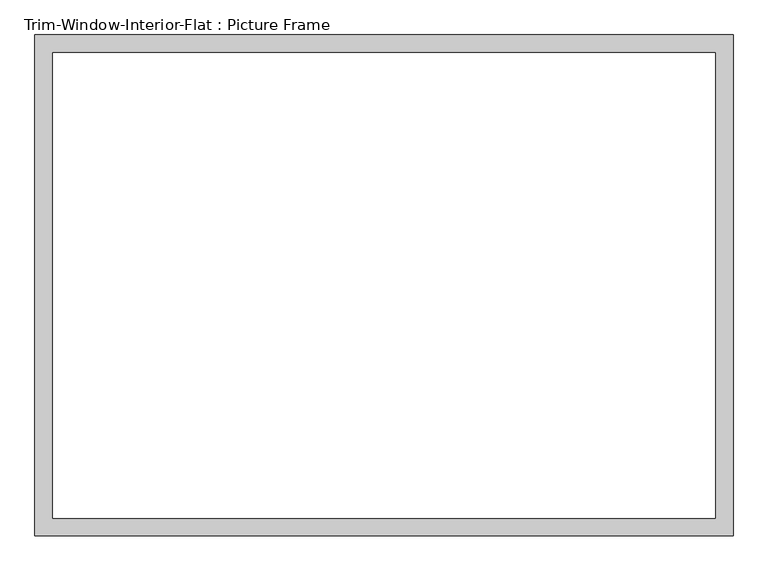
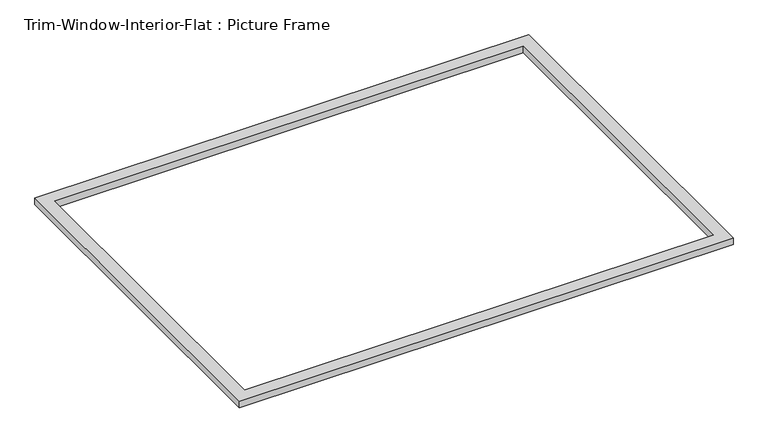
"""IFC4 building model written with IfcOpenShell, lengths in millimetres: proxy geometry, Trim-Window-Interior-Flat : Picture Frame."""

from ifc_helpers import new_model, si_unit, origin, origin_with_axes, place, context, project, spatial, polyline, outline, extrude, source, transform, mapped, element, save


def trim_window_interior_flat_picture_frame_12843d3c(model_context):
    return source(origin(), model_context, "Body", "SweptSolid", [
        extrude(outline(polyline([(1123.95, 44.45), (1123.95, -1568.45), (-1123.95, -1568.45), (-1123.95, 44.45), (1123.95, 44.45)]), holes=[polyline([(1066.8, -12.7), (-1066.8, -12.7), (-1066.8, -1511.3), (1066.8, -1511.3), (1066.8, -12.7)])]), origin_with_axes(), (0.0, 0.0, 1.0), 31.75),
    ])


if __name__ == "__main__":
    model = new_model("IFC4")
    model_context = context("Model", 3, world=origin())
    ifc_project = project(units=[si_unit("LENGTHUNIT", "METRE", prefix="MILLI")], contexts=[model_context])
    site = spatial("IfcSite", under=ifc_project)
    building = spatial("IfcBuilding", under=site)
    placement = place(None, origin())
    trim_window_interior_flat_picture_frame_shape = trim_window_interior_flat_picture_frame_12843d3c(model_context)
    element("IfcBuildingElementProxy", 1, Name="Trim-Window-Interior-Flat : Picture Frame", ObjectType="Trim-Window-Interior-Flat : Picture Frame", at=placement, inside=building, context=model_context, shape_type="MappedRepresentation", body=[
        mapped(trim_window_interior_flat_picture_frame_shape, transform((0.0, 0.0, 0.0), x_axis=(1.0, 0.0, 0.0), y_axis=(0.0, 1.0, 0.0), z_axis=(0.0, 0.0, 1.0))),
    ])
    save(model, "model.ifc")

# Revit data of these elements
# Type "Trim-Window-Interior-Flat : Picture Frame"
#   Trim Thickness_Picture Frame = 0' - 1 1/4"
#   Trim Width = 0' - 2 1/4"
#   Trim Thickness_with Sill = 0' - 0 3/4"
#   Sill Thickness = 0' - 1 1/4"
#   Opening Width [instance default] = 2' - 0"
#   Opening Height [instance default] = 3' - 0"
#   Default Elevation = 4' - 0"
#   Sill = no
#   Picture Frame = yes
#   Trim Material [instance default] = none
# Element 1 (IfcBuildingElementProxy, "Trim-Window-Interior-Flat : Picture Frame")
#   Opening Width = 7' - 1"
#   Opening Height = 5' - 0"
#   Trim Material = Wood - Stained
#   Materials on its faces: "Wood - Stained"
# Materials
#   "Wood - Stained": class "Wood", colour RGB 224 178 126, transparency 0, Cost = 0
